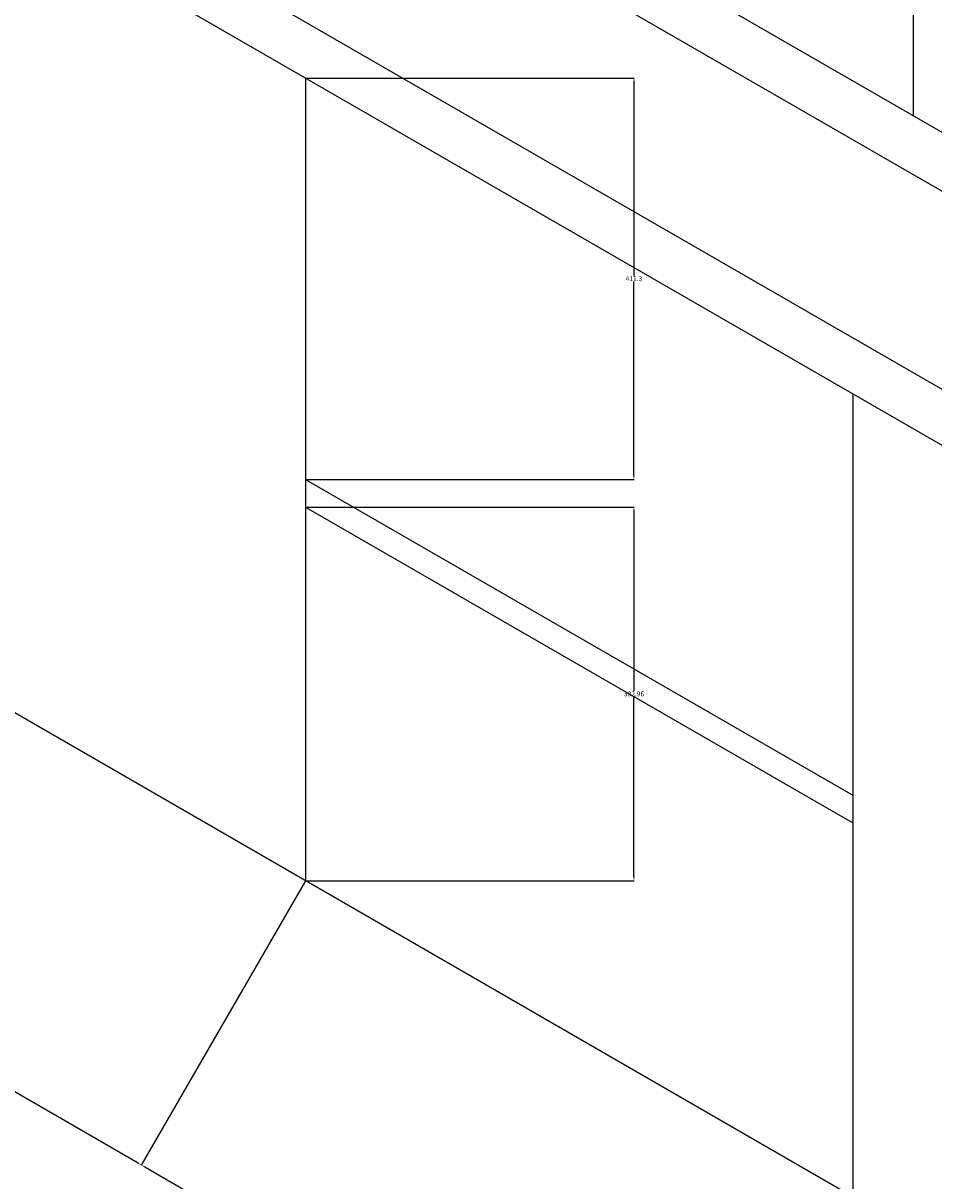
# Model space of a CAD drawing. Units: metres. Extents: x -2391 to 4922, y -635 to 4845.
# Tile 30 of 37: x 1265 to 2198, y 1238 to 2425. Entities that reach past the tile are written whole.
import ezdxf

# ---------------------------------------------------------------- set-up
doc = ezdxf.new("R2010")
doc.units = ezdxf.units.M
doc.header["$MEASUREMENT"] = 0
for name, color, linetype, lineweight in [('A-ANNO-DIMS', 2, 'Continuous', 18), ('A-FLOR-FIXT', 3, 'Continuous', 25), ('A-GLAZ', 4, 'Continuous', 25)]:
    doc.layers.add(name, color=color, linetype=linetype, lineweight=lineweight)
doc.styles.get("Standard").update_dxf_attribs({"font": 'arial.ttf'})
doc.dimstyles.get("Standard").update_dxf_attribs({"dimtxt": 5, "dimasz": 4, "dimexe": 0.18, "dimexo": 0.0625, "dimgap": 0.09, "dimtad": 0, "dimtih": 1, "dimtoh": 1, "dimdec": 0, "dimzin": 0, "dimdsep": 46, "dimtxsty": 'Standard', "dimcen": 0.09, "dimadec": 0, "dimazin": 0, "dimtfac": 1, "dimtdec": 0, "dimtofl": 0, "dimtmove": 0, "dimatfit": 3, "dimfxl": 1, "dimtolj": 1, "dimtzin": 0, "dimarcsym": 0})

# ---------------------------------------------------------------- blocks, each defined once
blk = doc.blocks.new('*D8')
at = {"layer": 'A-ANNO-DIMS', "color": 0, "lineweight": -2, "transparency": 16777216}
for p, q in [((-2047.3, 3005.2), (-2047.3, -631.4)), ((4577.8, 2350.2), (4577.8, -631.4)), ((-2043.3, -631.2), (1257.6, -631.2)), ((4573.8, -631.2), (1272.8, -631.2))]:
    blk.add_line(p, q, dxfattribs=at)
at = {"layer": 'A-ANNO-DIMS', "color": 0, "transparency": 16777216}
for points in [[(-2043.3, -630.6), (-2043.3, -631.9), (-2047.3, -631.2)], [(4573.8, -630.6), (4573.8, -631.9), (4577.8, -631.2)]]:
    blk.add_solid(points, dxfattribs=at)
at = {"layer": 'Defpoints', "color": 0, "transparency": 16777216}
for p in [(-2047.3, 3005.3), (4577.8, 2350.3), (4577.8, -631.2)]:
    blk.add_point(p, dxfattribs=at)
at = {"layer": 'A-ANNO-DIMS', "color": 0, "transparency": 16777216, "insert": (1265.2, -631.2), "char_height": 5, "attachment_point": 5}
blk.add_mtext('\\A1;6625', dxfattribs=at)
blk = doc.blocks.new('*D19')
at = {"layer": 'A-ANNO-DIMS', "color": 0, "lineweight": -2, "transparency": 16777216}
for p, q in [((994.5, 1869), (826.2, 1577.5)), ((829.7, 1575.6), (1101.7, 1418.6)), ((1554.6, 1545.6), (1386.3, 1254.1)), ((1382.9, 1256.3), (1110.9, 1413.3))]:
    blk.add_line(p, q, dxfattribs=at)
at = {"layer": 'A-ANNO-DIMS', "color": 0, "transparency": 16777216}
for points in [[(830.1, 1576.2), (829.4, 1575.1), (826.3, 1577.6)], [(1383.2, 1256.8), (1382.6, 1255.7), (1386.4, 1254.3)]]:
    blk.add_solid(points, dxfattribs=at)
at = {"layer": 'Defpoints', "color": 0, "transparency": 16777216}
for p in [(994.5, 1869.1), (826.3, 1577.6), (1554.6, 1545.7)]:
    blk.add_point(p, dxfattribs=at)
at = {"layer": 'A-ANNO-DIMS', "color": 0, "transparency": 16777216, "insert": (1106.3, 1416), "char_height": 5, "attachment_point": 5}
blk.add_mtext('\\A1;646.8', dxfattribs=at)
blk = doc.blocks.new('*D20')
at = {"layer": 'A-ANNO-DIMS', "color": 0, "lineweight": -2, "transparency": 16777216}
for p, q in [((1554.6, 1545.6), (1386.3, 1254.1)), ((1389.8, 1252.3), (1662.1, 1095.1)), ((2115.2, 1222), (1946.9, 930.4)), ((1943.5, 932.6), (1671.3, 1089.8))]:
    blk.add_line(p, q, dxfattribs=at)
at = {"layer": 'A-ANNO-DIMS', "color": 0, "transparency": 16777216}
for points in [[(1390.2, 1252.8), (1389.5, 1251.7), (1386.4, 1254.3)], [(1943.9, 933.2), (1943.2, 932), (1947, 930.6)]]:
    blk.add_solid(points, dxfattribs=at)
at = {"layer": 'Defpoints', "color": 0, "transparency": 16777216}
for p in [(1554.6, 1545.7), (1386.4, 1254.3), (2115.2, 1222)]:
    blk.add_point(p, dxfattribs=at)
at = {"layer": 'A-ANNO-DIMS', "color": 0, "transparency": 16777216, "insert": (1666.7, 1092.4), "char_height": 5, "attachment_point": 5}
blk.add_mtext('\\A1;647.3', dxfattribs=at)
blk = doc.blocks.new('*D25')
at = {"layer": 'A-ANNO-DIMS', "color": 0, "lineweight": -2, "transparency": 16777216}
for p, q in [((1554.7, 2368.3), (1891.3, 2368.3)), ((1891.1, 2364.3), (1891.1, 2165.3)), ((1891.1, 1961), (1891.1, 2160)), ((1554.7, 1957), (1891.3, 1957))]:
    blk.add_line(p, q, dxfattribs=at)
at = {"layer": 'A-ANNO-DIMS', "color": 0, "transparency": 16777216}
for points in [[(1890.4, 2364.3), (1891.8, 2364.3), (1891.1, 2368.3)], [(1890.4, 1961), (1891.8, 1961), (1891.1, 1957)]]:
    blk.add_solid(points, dxfattribs=at)
at = {"layer": 'Defpoints', "color": 0, "transparency": 16777216}
for p in [(1554.6, 2368.3), (1554.6, 1957), (1891.1, 1957)]:
    blk.add_point(p, dxfattribs=at)
at = {"layer": 'A-ANNO-DIMS', "color": 0, "transparency": 16777216, "insert": (1891.1, 2162.7), "char_height": 5, "attachment_point": 5}
blk.add_mtext('\\A1;411.3', dxfattribs=at)
blk = doc.blocks.new('*D26')
at = {"layer": 'A-ANNO-DIMS', "color": 0, "lineweight": -2, "transparency": 16777216}
for p, q in [((1554.7, 1928.6), (1891.3, 1928.6)), ((1891.1, 1924.6), (1891.1, 1739.8)), ((1891.1, 1549.7), (1891.1, 1734.5)), ((1554.7, 1545.7), (1891.3, 1545.7))]:
    blk.add_line(p, q, dxfattribs=at)
at = {"layer": 'A-ANNO-DIMS', "color": 0, "transparency": 16777216}
for points in [[(1890.4, 1924.6), (1891.8, 1924.6), (1891.1, 1928.6)], [(1890.4, 1549.7), (1891.8, 1549.7), (1891.1, 1545.7)]]:
    blk.add_solid(points, dxfattribs=at)
at = {"layer": 'Defpoints', "color": 0, "transparency": 16777216}
for p in [(1554.6, 1928.6), (1554.6, 1545.7), (1891.1, 1545.7)]:
    blk.add_point(p, dxfattribs=at)
at = {"layer": 'A-ANNO-DIMS', "color": 0, "transparency": 16777216, "insert": (1891.1, 1737.2), "char_height": 5, "attachment_point": 5}
blk.add_mtext('\\A1;382.96', dxfattribs=at)

msp = doc.modelspace()

# ---------------------------------------------------------------- linework, layer by layer
at = {"layer": 'A-FLOR-FIXT'}
for p, q in [((550.7419, 3005.2763), (3148.8181, 1505.2763)), ((546.8938, 2950.1416), (3148.8181, 1447.9199)), ((1554.6155, 2368.3332), (1554.6155, 1545.6896)), ((3148.8181, 625.2763), (550.7419, 2125.2763)), ((2115.2362, 2044.6587), (2115.2362, 1222.0151)), ((1554.6155, 1957.0114), (2115.2362, 1633.3369)), ((1554.6155, 1928.6456), (2115.2362, 1604.9711))]:
    msp.add_line(p, q, dxfattribs=at)
at = {"layer": 'A-GLAZ'}
for p, q in [((2177.2021, 3114.7443), (2177.2021, 2329.8889)), ((1573.5273, 2678.4207), (2820.8768, 1958.2631)), ((2891.4324, 1856.8211), (1496.0309, 2662.4566))]:
    msp.add_line(p, q, dxfattribs=at)

# ---------------------------------------------------------------- dimensions: what is measured, and where the dimension line sits
at = {"layer": 'A-ANNO-DIMS'}
dim = msp.add_linear_dim(base=(4577.76, -631.2237), p1=(-2047.3343, 3005.2763), p2=(4577.76, 2350.2763), dimstyle='Standard', override={"dimdec": 0, "dimlfac": 1, "dimrnd": 0, "dimzin": 0, "dimdsep": 46, "dimlunit": 2}, dxfattribs=at)
dim.commit()
dim.dimension.update_dxf_attribs({"geometry": '*D8', "text_midpoint": (1265.2128, -631.2237)})
for base, p1, p2, angle, override, picture, middle in [((1891.1155, 1957.0114), (1554.6155, 2368.3332), (1554.6155, 1957.0114), 270, {"dimdec": 1, "dimlfac": 1, "dimrnd": 0, "dimzin": 0, "dimdsep": 46, "dimlunit": 2}, '*D25', (1891.1155, 2162.6723)), ((1891.1155, 1545.6896), (1554.6155, 1928.6456), (1554.6155, 1545.6896), 270, {"dimdec": 2, "dimlfac": 1, "dimrnd": 0, "dimzin": 0, "dimdsep": 46, "dimlunit": 2}, '*D26', (1891.1155, 1737.1676)), ((826.2603, 1577.6489), (1554.6155, 1545.6896), (994.5103, 1869.0664), 150, {"dimdec": 1, "dimlfac": 1, "dimrnd": 0, "dimzin": 0, "dimdsep": 46, "dimlunit": 2}, '*D19', (1106.3129, 1415.9604)), ((1386.3655, 1254.272), (2115.2362, 1222.0151), (1554.6155, 1545.6896), 150, {"dimdec": 1, "dimlfac": 1, "dimrnd": 0, "dimzin": 0, "dimdsep": 46, "dimlunit": 2}, '*D20', (1666.6758, 1092.4348))]:
    dim = msp.add_linear_dim(base=base, p1=p1, p2=p2, angle=angle, dimstyle='Standard', override=override, dxfattribs=at)
    dim.commit()
    dim.dimension.update_dxf_attribs({"geometry": picture, "text_midpoint": middle})

doc.saveas('drawing.dxf')
